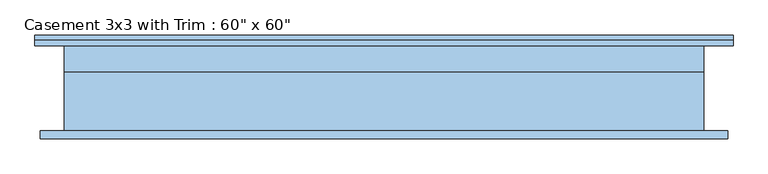
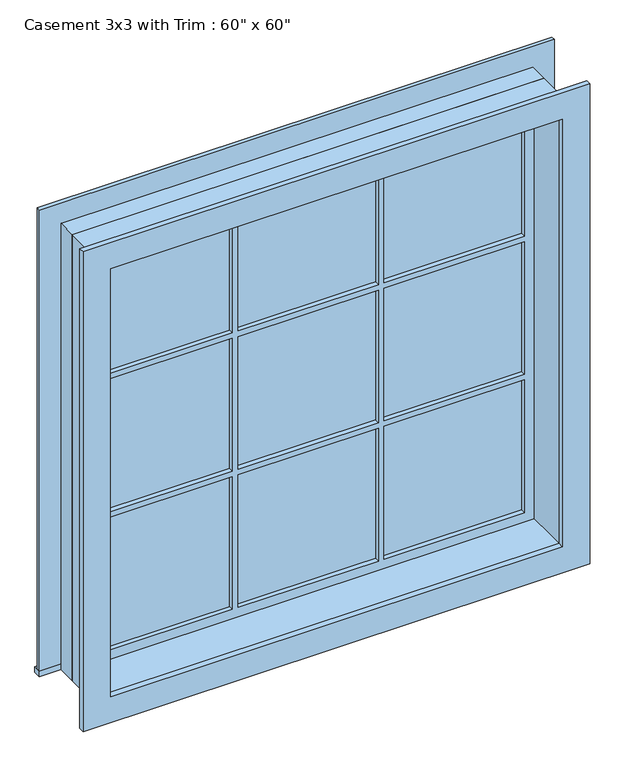
"""IFC4 building model written with IfcOpenShell, lengths in millimetres: window geometry."""

from ifc_helpers import new_model, si_unit, frame, origin, place, context, project, spatial, polyline, outline, extrude, source, transform, mapped, element, save


def window_9e391526(model_context):
    return source(origin(), model_context, "Body", "SweptSolid", [
        extrude(outline(polyline([(-831.85, 127.0), (831.85, 127.0), (831.85, 101.6), (-831.85, 101.6), (-831.85, 127.0)])), frame((0.0, 0.0, 914.4), z_axis=(0.0, 0.0, 1.0), x_axis=(1.0, 0.0, 0.0)), (0.0, 0.0, 1.0), 19.05),
        extrude(outline(polyline([(2419.35, -742.95), (2419.35, 742.95), (933.45, 742.95), (933.45, 831.85), (2508.25, 831.85), (2508.25, -831.85), (933.45, -831.85), (933.45, -742.95), (2419.35, -742.95)])), frame((0.0, 101.6, 0.0), z_axis=(0.0, 1.0, 0.0), x_axis=(0.0, 0.0, 1.0)), (0.0, 0.0, 1.0), 12.7),
        extrude(outline(polyline([(245.5333333, 66.675), (698.5, 66.675), (698.5, 53.975), (245.5333333, 53.975), (245.5333333, 66.675)])), frame((0.0, 0.0, 1921.9333333), z_axis=(0.0, 0.0, 1.0), x_axis=(1.0, 0.0, 0.0)), (0.0, 0.0, 1.0), 452.9666667),
        extrude(outline(polyline([(-226.4833333, 66.675), (226.4833333, 66.675), (226.4833333, 53.975), (-226.4833333, 53.975), (-226.4833333, 66.675)])), frame((0.0, 0.0, 1921.9333333), z_axis=(0.0, 0.0, 1.0), x_axis=(1.0, 0.0, 0.0)), (0.0, 0.0, 1.0), 452.9666667),
        extrude(outline(polyline([(-698.5, 66.675), (-245.5333333, 66.675), (-245.5333333, 53.975), (-698.5, 53.975), (-698.5, 66.675)])), frame((0.0, 0.0, 1921.9333333), z_axis=(0.0, 0.0, 1.0), x_axis=(1.0, 0.0, 0.0)), (0.0, 0.0, 1.0), 452.9666667),
        extrude(outline(polyline([(-698.5, 66.675), (-245.5333333, 66.675), (-245.5333333, 53.975), (-698.5, 53.975), (-698.5, 66.675)])), frame((0.0, 0.0, 1449.9166667), z_axis=(0.0, 0.0, 1.0), x_axis=(1.0, 0.0, 0.0)), (0.0, 0.0, 1.0), 452.9666667),
        extrude(outline(polyline([(-226.4833333, 66.675), (226.4833333, 66.675), (226.4833333, 53.975), (-226.4833333, 53.975), (-226.4833333, 66.675)])), frame((0.0, 0.0, 1449.9166667), z_axis=(0.0, 0.0, 1.0), x_axis=(1.0, 0.0, 0.0)), (0.0, 0.0, 1.0), 452.9666667),
        extrude(outline(polyline([(245.5333333, 66.675), (698.5, 66.675), (698.5, 53.975), (245.5333333, 53.975), (245.5333333, 66.675)])), frame((0.0, 0.0, 1449.9166667), z_axis=(0.0, 0.0, 1.0), x_axis=(1.0, 0.0, 0.0)), (0.0, 0.0, 1.0), 452.9666667),
        extrude(outline(polyline([(245.5333333, 66.675), (698.5, 66.675), (698.5, 53.975), (245.5333333, 53.975), (245.5333333, 66.675)])), frame((0.0, 0.0, 977.9), z_axis=(0.0, 0.0, 1.0), x_axis=(1.0, 0.0, 0.0)), (0.0, 0.0, 1.0), 452.9666667),
        extrude(outline(polyline([(-226.4833333, 66.675), (226.4833333, 66.675), (226.4833333, 53.975), (-226.4833333, 53.975), (-226.4833333, 66.675)])), frame((0.0, 0.0, 977.9), z_axis=(0.0, 0.0, 1.0), x_axis=(1.0, 0.0, 0.0)), (0.0, 0.0, 1.0), 452.9666667),
        extrude(outline(polyline([(-698.5, 66.675), (-245.5333333, 66.675), (-245.5333333, 53.975), (-698.5, 53.975), (-698.5, 66.675)])), frame((0.0, 0.0, 977.9), z_axis=(0.0, 0.0, 1.0), x_axis=(1.0, 0.0, 0.0)), (0.0, 0.0, 1.0), 452.9666667),
        extrude(outline(polyline([(2495.55, 819.15), (2495.55, -819.15), (857.25, -819.15), (857.25, 819.15), (2495.55, 819.15)]), holes=[polyline([(2406.65, 730.25), (946.15, 730.25), (946.15, -730.25), (2406.65, -730.25), (2406.65, 730.25)])]), frame((0.0, -120.65, 0.0), z_axis=(0.0, 1.0, 0.0), x_axis=(0.0, 0.0, 1.0)), (0.0, 0.0, 1.0), 19.05),
        extrude(outline(polyline([(2419.35, -742.95), (933.45, -742.95), (933.45, 742.95), (2419.35, 742.95), (2419.35, -742.95)]), holes=[polyline([(2374.9, -245.5333333), (1921.9333333, -245.5333333), (1921.9333333, -698.5), (2374.9, -698.5), (2374.9, -245.5333333)]), polyline([(1902.8833333, -245.5333333), (1449.9166667, -245.5333333), (1449.9166667, -698.5), (1902.8833333, -698.5), (1902.8833333, -245.5333333)]), polyline([(1430.8666667, -245.5333333), (977.9, -245.5333333), (977.9, -698.5), (1430.8666667, -698.5), (1430.8666667, -245.5333333)]), polyline([(2374.9, 226.4833333), (1921.9333333, 226.4833333), (1921.9333333, -226.4833333), (2374.9, -226.4833333), (2374.9, 226.4833333)]), polyline([(1902.8833333, 226.4833333), (1449.9166667, 226.4833333), (1449.9166667, -226.4833333), (1902.8833333, -226.4833333), (1902.8833333, 226.4833333)]), polyline([(1430.8666667, 226.4833333), (977.9, 226.4833333), (977.9, -226.4833333), (1430.8666667, -226.4833333), (1430.8666667, 226.4833333)]), polyline([(2374.9, 698.5), (1921.9333333, 698.5), (1921.9333333, 245.5333333), (2374.9, 245.5333333), (2374.9, 698.5)]), polyline([(1902.8833333, 698.5), (1449.9166667, 698.5), (1449.9166667, 245.5333333), (1902.8833333, 245.5333333), (1902.8833333, 698.5)]), polyline([(1430.8666667, 698.5), (977.9, 698.5), (977.9, 245.5333333), (1430.8666667, 245.5333333), (1430.8666667, 698.5)])]), frame((0.0, 38.1, 0.0), z_axis=(0.0, 1.0, 0.0), x_axis=(0.0, 0.0, 1.0)), (0.0, 0.0, 1.0), 44.45),
        extrude(outline(polyline([(2438.4, -762.0), (914.4, -762.0), (914.4, 762.0), (2438.4, 762.0), (2438.4, -762.0)]), holes=[polyline([(2406.65, -730.25), (2406.65, 730.25), (946.15, 730.25), (946.15, -730.25), (2406.65, -730.25)])]), frame((0.0, -101.6, 0.0), z_axis=(0.0, 1.0, 0.0), x_axis=(0.0, 0.0, 1.0)), (0.0, 0.0, 1.0), 139.7),
        extrude(outline(polyline([(2438.4, 762.0), (2438.4, -762.0), (914.4, -762.0), (914.4, 762.0), (2438.4, 762.0)]), holes=[polyline([(2419.35, 742.95), (933.45, 742.95), (933.45, -742.95), (2419.35, -742.95), (2419.35, 742.95)])]), frame((0.0, 38.1, 0.0), z_axis=(0.0, 1.0, 0.0), x_axis=(0.0, 0.0, 1.0)), (0.0, 0.0, 1.0), 63.5),
    ])


if __name__ == "__main__":
    model = new_model("IFC4")
    model_context = context("Model", 3, world=origin())
    ifc_project = project(units=[si_unit("LENGTHUNIT", "METRE", prefix="MILLI")], contexts=[model_context])
    site = spatial("IfcSite", under=ifc_project)
    building = spatial("IfcBuilding", under=site)
    placement = place(None, origin())
    window_shape = window_9e391526(model_context)
    element("IfcWindow", 1, ObjectType="Casement 3x3 with Trim : 60\" x 60\"", at=placement, inside=building, context=model_context, shape_type="MappedRepresentation", body=[
        mapped(window_shape, transform((0.0, 0.0, 0.0), x_axis=(1.0, 0.0, 0.0), y_axis=(0.0, 1.0, 0.0), z_axis=(0.0, 0.0, 1.0))),
    ])
    save(model, "model.ifc")

# Revit data of these elements
# Type "Casement 3x3 with Trim : 60\" x 60\""
#   Type Mark = "13"
#   Construction Type Id = "GSP4R"
#   Assembly Code = "B2020100"
#   Analytic Construction = "1/8 in Pilkington single glazing"
#   Visual Light Transmittance = 0.9
#   Solar Heat Gain Coefficient = 0.78
#   Heat Transfer Coefficient (U) = 0.6496 BTU/(h·ft²·°F)
#   Height = 5' - 0"
#   Default Sill Height = 3' - 0"
#   Trim Projection - Ext. = 0' - 0 1/2"
#   Trim Projection - Int. = 0' - 0 3/4"
#   Trim Width - Exterior = 0' - 3 1/2"
#   Trim Width - Interior = 0' - 3 1/2"
#   Width = 5' - 0"
#   Window Inset = 0' - 0 3/4"
#   Define Thermal Properties by = 1
#   Glass Pane Material = Glass
#   Sash Material = Sash
#   Trim Exterior Material = Trim
#   Trim Interior Material = Trim
#   Wall Closure = (empty or 0)
# Element 1 (IfcWindow, "Casement 3x3 with Trim : 60\" x 60\"")
#   Materials on its faces: "Sash", "Glass", "Trim"
# Materials
#   "Glass": class "Glass", colour RGB 0 128 192, transparency 0.75, Description = "Soda Lime Glass", Cost = 0
#   "Sash": class "Wood", colour RGB 224 178 126, transparency 0
#   "Trim": class "Wood", colour RGB 224 178 126, transparency 0
